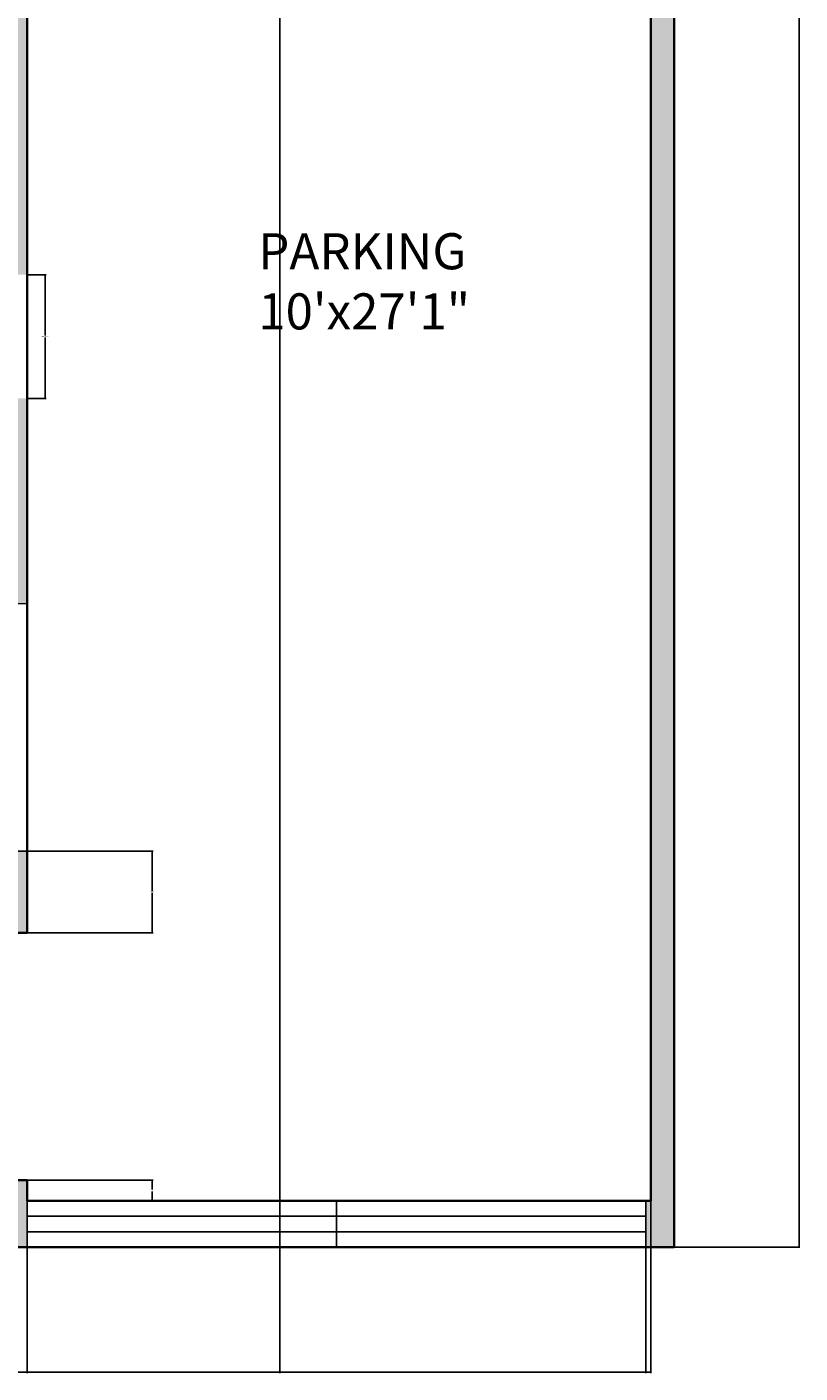
# Model space of a CAD drawing. Units: millimetres. Extents: x 2817 to 5038, y 1110 to 3565.
# Tile 9 of 21: x 3061 to 3211, y 1110 to 1371. Entities that reach past the tile are written whole.
import ezdxf

# ---------------------------------------------------------------- set-up
doc = ezdxf.new("R2010")
doc.units = ezdxf.units.MM
for name, color, linetype, lineweight in [('A-ANNO-DIMS', 2, 'Continuous', 18), ('A-AREA-IDEN', 7, 'Continuous', 18), ('A-WALL', 7, 'Continuous', 35), ('DOOR&WINDOW', 1, 'Continuous', 25)]:
    doc.layers.add(name, color=color, linetype=linetype, lineweight=lineweight)
doc.layers.add('A-WALL-PATT', color=51, linetype='Continuous', lineweight=13, true_color=0xf7f281)
doc.styles.get("Standard").update_dxf_attribs({"font": 'arial.ttf'})
doc.dimstyles.get("Standard").update_dxf_attribs({"dimtxt": 0.18, "dimasz": 0.18, "dimexe": 0.18, "dimexo": 0.0625, "dimgap": 0.09, "dimtad": 0, "dimtih": 1, "dimtoh": 1, "dimdec": 4, "dimzin": 0, "dimdsep": 46, "dimtxsty": 'Standard', "dimcen": 0.09, "dimadec": 0, "dimazin": 0, "dimtfac": 1, "dimtdec": 4, "dimtofl": 0, "dimtmove": 0, "dimatfit": 3, "dimfxl": 1, "dimtolj": 1, "dimtzin": 0, "dimarcsym": 0})

# ---------------------------------------------------------------- blocks, each defined once
blk = doc.blocks.new('WIN-4FT')
for p, q in [((0, 47.85), (9, 48)), ((0, 0), (0, 47.85)), ((3, 0), (3, 47.85)), ((6, 48), (6, 0)), ((9, 48), (9, 0)), ((9, 0), (0, 0))]:
    blk.add_line(p, q)
blk = doc.blocks.new('*D16')
at = {"layer": 'A-ANNO-DIMS', "color": 0, "lineweight": -2, "transparency": 16777216}
for p, q in [((3061.2, 1323.1), (3064.92, 1323.1)), ((3064.74, 1322.92), (3064.74, 1311.28)), ((3064.74, 1299.28), (3064.74, 1310.92)), ((3061.2, 1299.1), (3064.92, 1299.1))]:
    blk.add_line(p, q, dxfattribs=at)
for points in [[(3064.71, 1322.92), (3064.77, 1322.92), (3064.74, 1323.1)], [(3064.71, 1299.28), (3064.77, 1299.28), (3064.74, 1299.1)]]:
    blk.add_solid(points, dxfattribs=at)
at = {"layer": 'Defpoints', "color": 0, "lineweight": -2, "transparency": 16777216}
for p in [(3061.14, 1323.1), (3064.74, 1323.1), (3061.14, 1299.1)]:
    blk.add_point(p, dxfattribs=at)
at = {"layer": 'A-ANNO-DIMS', "color": 0, "transparency": 16777216, "insert": (3064.74, 1311.1), "char_height": 0.18, "attachment_point": 5}
blk.add_mtext('\\A1;WIN. 24 TYP.', dxfattribs=at)
blk = doc.blocks.new('*D27')
at = {"layer": 'A-ANNO-DIMS', "color": 0, "lineweight": -2, "transparency": 16777216}
for p, q in [((3186.8, 1614.44), (3211.17, 1614.44)), ((3210.99, 1614.26), (3210.99, 1374.62)), ((3210.99, 1134.62), (3210.99, 1374.25)), ((3186.8, 1134.44), (3211.17, 1134.44))]:
    blk.add_line(p, q, dxfattribs=at)
for points in [[(3210.96, 1614.26), (3211.02, 1614.26), (3210.99, 1614.44)], [(3210.96, 1134.62), (3211.02, 1134.62), (3210.99, 1134.44)]]:
    blk.add_solid(points, dxfattribs=at)
at = {"layer": 'Defpoints', "color": 0, "lineweight": -2, "transparency": 16777216}
for p in [(3186.74, 1614.44), (3210.99, 1614.44), (3186.74, 1134.44)]:
    blk.add_point(p, dxfattribs=at)
at = {"layer": 'A-ANNO-DIMS', "color": 0, "transparency": 16777216, "insert": (3210.99, 1374.44), "char_height": 0.18, "attachment_point": 5}
blk.add_mtext('\\A1;480', dxfattribs=at)
blk = doc.blocks.new('*D28')
at = {"layer": 'A-ANNO-DIMS', "color": 0, "lineweight": -2, "transparency": 16777216}
for p, q in [((2841.74, 1134.37), (2841.74, 1110.01)), ((3061.24, 1134.37), (3061.24, 1110.01)), ((2841.92, 1110.19), (2951.09, 1110.19)), ((3061.06, 1110.19), (2951.89, 1110.19))]:
    blk.add_line(p, q, dxfattribs=at)
for points in [[(2841.92, 1110.22), (2841.92, 1110.16), (2841.74, 1110.19)], [(3061.06, 1110.22), (3061.06, 1110.16), (3061.24, 1110.19)]]:
    blk.add_solid(points, dxfattribs=at)
at = {"layer": 'Defpoints', "color": 0, "lineweight": -2, "transparency": 16777216}
for p in [(2841.74, 1134.44), (3061.24, 1134.44), (3061.24, 1110.19)]:
    blk.add_point(p, dxfattribs=at)
at = {"layer": 'A-ANNO-DIMS', "color": 0, "transparency": 16777216, "insert": (2951.49, 1110.19), "char_height": 0.18, "attachment_point": 5}
blk.add_mtext('\\A1;219.5', dxfattribs=at)
blk = doc.blocks.new('*D29')
at = {"layer": 'A-ANNO-DIMS', "color": 0, "lineweight": -2, "transparency": 16777216}
for p, q in [((3061.24, 1134.37), (3061.24, 1110.01)), ((3181.24, 1134.37), (3181.24, 1110.01)), ((3061.42, 1110.19), (3120.96, 1110.19)), ((3181.06, 1110.19), (3121.52, 1110.19))]:
    blk.add_line(p, q, dxfattribs=at)
for points in [[(3061.42, 1110.22), (3061.42, 1110.16), (3061.24, 1110.19)], [(3181.06, 1110.22), (3181.06, 1110.16), (3181.24, 1110.19)]]:
    blk.add_solid(points, dxfattribs=at)
at = {"layer": 'Defpoints', "color": 0, "lineweight": -2, "transparency": 16777216}
for p in [(3061.24, 1134.44), (3181.24, 1134.44), (3181.24, 1110.19)]:
    blk.add_point(p, dxfattribs=at)
at = {"layer": 'A-ANNO-DIMS', "color": 0, "transparency": 16777216, "insert": (3121.24, 1110.19), "char_height": 0.18, "attachment_point": 5}
blk.add_mtext('\\A1;120', dxfattribs=at)
blk = doc.blocks.new('*D37')
at = {"layer": 'A-ANNO-DIMS', "color": 0, "lineweight": -2, "transparency": 16777216}
for p, q in [((3110.24, 1473.37), (3110.24, 1110.01)), ((3182.24, 1473.37), (3182.24, 1110.01)), ((3110.42, 1110.19), (3146.02, 1110.19)), ((3182.06, 1110.19), (3146.46, 1110.19))]:
    blk.add_line(p, q, dxfattribs=at)
for points in [[(3110.42, 1110.22), (3110.42, 1110.16), (3110.24, 1110.19)], [(3182.06, 1110.22), (3182.06, 1110.16), (3182.24, 1110.19)]]:
    blk.add_solid(points, dxfattribs=at)
at = {"layer": 'Defpoints', "color": 0, "lineweight": -2, "transparency": 16777216}
for p in [(3110.24, 1473.44), (3182.24, 1473.44), (3182.24, 1110.19)]:
    blk.add_point(p, dxfattribs=at)
at = {"layer": 'A-ANNO-DIMS', "color": 0, "transparency": 16777216, "insert": (3146.24, 1110.19), "char_height": 0.18, "attachment_point": 5}
blk.add_mtext('\\A1;72', dxfattribs=at)
blk = doc.blocks.new('*D48')
at = {"layer": 'A-ANNO-DIMS', "color": 0, "lineweight": -2, "transparency": 16777216}
for p, q in [((3061.3, 1211.29), (3085.67, 1211.29)), ((3085.49, 1211.11), (3085.49, 1203.54)), ((3085.49, 1195.62), (3085.49, 1203.18)), ((3061.3, 1195.44), (3085.67, 1195.44))]:
    blk.add_line(p, q, dxfattribs=at)
for points in [[(3085.46, 1211.11), (3085.52, 1211.11), (3085.49, 1211.29)], [(3085.46, 1195.62), (3085.52, 1195.62), (3085.49, 1195.44)]]:
    blk.add_solid(points, dxfattribs=at)
at = {"layer": 'Defpoints', "color": 0, "lineweight": -2, "transparency": 16777216}
for p in [(3061.24, 1211.29), (3061.24, 1195.44), (3085.49, 1195.44)]:
    blk.add_point(p, dxfattribs=at)
at = {"layer": 'A-ANNO-DIMS', "color": 0, "transparency": 16777216, "insert": (3085.49, 1203.36), "char_height": 0.18, "attachment_point": 5}
blk.add_mtext('\\A1;15.854', dxfattribs=at)
blk = doc.blocks.new('*D50')
at = {"layer": 'A-ANNO-DIMS', "color": 0, "lineweight": -2, "transparency": 16777216}
for p, q in [((3061.301815, 1147.435717), (3085.669315, 1147.435717)), ((3085.489315, 1147.255717), (3085.489315, 1145.615717)), ((3085.489315, 1143.615717), (3085.489315, 1145.255717)), ((3061.301815, 1143.435717), (3085.669315, 1143.435717))]:
    blk.add_line(p, q, dxfattribs=at)
for points in [[(3085.459315, 1147.255717), (3085.519315, 1147.255717), (3085.489315, 1147.435717)], [(3085.459315, 1143.615717), (3085.519315, 1143.615717), (3085.489315, 1143.435717)]]:
    blk.add_solid(points, dxfattribs=at)
at = {"layer": 'Defpoints', "color": 0, "lineweight": -2, "transparency": 16777216}
for p in [(3061.239315, 1147.435717), (3061.239315, 1143.435717), (3085.489315, 1143.435717)]:
    blk.add_point(p, dxfattribs=at)
at = {"layer": 'A-ANNO-DIMS', "color": 0, "transparency": 16777216, "insert": (3085.489315, 1145.435717), "char_height": 0.18, "attachment_point": 5}
blk.add_mtext('\\A1;4', dxfattribs=at)

msp = doc.modelspace()

# ---------------------------------------------------------------- hatches: boundary and pattern name
at = {"layer": 'A-WALL-PATT'}
h = msp.add_hatch(color=256, dxfattribs=at)
h.dxf.hatch_style = 1
h.paths.add_polyline_path([(3186.7393, 1614.4357), (2841.7393, 1614.4357), (2841.7393, 1568.614), (2850.7393, 1568.7609), (2850.7393, 1605.4357), (2982.7393, 1605.4357), (2991.7393, 1605.4357), (3052.2393, 1605.4357), (3052.2393, 1573.7835), (3061.2393, 1573.7835), (3061.2393, 1605.4357), (3182.2393, 1605.4357), (3182.2393, 1143.4357), (3181.2393, 1143.4357), (3181.2393, 1134.4357), (3186.7393, 1134.4357)])
h.paths.add_polyline_path([(3061.2393, 1143.4357), (3061.2393, 1147.4357), (3052.2393, 1147.4357), (3052.2393, 1143.4357), (2850.7393, 1143.4357), (2850.7393, 1145.2996), (2841.7393, 1145.2996), (2841.7393, 1134.4357), (3061.2393, 1134.4357)], flags=17)
h.paths.add_polyline_path([(2850.7393, 1265.4357), (2946.7393, 1265.4357), (2946.7393, 1270.8357), (2946.7393, 1274.4357), (2850.7393, 1274.4357), (2850.7381, 1274.4357), (2850.7381, 1274.2564), (2841.7393, 1274.2564), (2841.7393, 1193.1527), (2850.7393, 1193.2996)], flags=17)
h.paths.add_polyline_path([(3061.2393, 1299.098), (3052.2393, 1299.098), (3052.2393, 1274.4357), (2991.7393, 1274.4357), (2991.7393, 1340.4357), (2982.7393, 1340.4357), (2982.7393, 1274.4357), (2982.7393, 1265.4357), (3052.2393, 1265.4357), (3052.2393, 1259.143), (3061.2393, 1259.2899)], flags=17)
h.paths.add_polyline_path([(3061.2393, 1383.4357), (3052.2393, 1383.4357), (3052.2393, 1379.4357), (2931.7393, 1379.4357), (2922.7393, 1379.4357), (2850.7393, 1379.4357), (2850.7381, 1379.4357), (2850.7381, 1379.3646), (2841.7393, 1379.3646), (2841.7393, 1322.1095), (2850.7393, 1322.2564), (2850.7393, 1370.4357), (2982.7393, 1370.4357), (2987.2393, 1370.4357), (3017.2393, 1370.4357), (3052.2393, 1370.4357), (3052.2393, 1323.098), (3061.2393, 1323.098)], flags=17)
h = msp.add_hatch(color=256, dxfattribs=at)
h.dxf.hatch_style = 1
h.paths.add_polyline_path([(3061.2393, 1549.7835), (3052.2393, 1549.7835), (3052.2393, 1509.4357), (2991.7393, 1509.4357), (2991.7393, 1575.4357), (2982.7393, 1575.4357), (2982.7393, 1509.4357), (2982.7393, 1500.4357), (3052.2393, 1500.4357), (3052.2393, 1498.4661), (3061.2393, 1498.613)])
h.paths.add_polyline_path([(2946.7393, 1505.8357), (2946.7393, 1509.4357), (2850.7393, 1509.4357), (2850.7393, 1520.7609), (2841.7393, 1520.7609), (2841.7393, 1427.2177), (2850.7393, 1427.3646), (2850.7393, 1500.4357), (2922.7393, 1500.4357), (2931.7393, 1500.4357), (2946.7393, 1500.4357)])
h.paths.add_polyline_path([(3061.2393, 1450.613), (3052.2393, 1450.613), (3052.2393, 1431.4357), (3059.4393, 1431.4357), (3061.2393, 1431.4357)])
h.paths.add_polyline_path([(3061.2393, 1211.2899), (3052.2393, 1211.2899), (3052.2393, 1195.4357), (3059.4393, 1195.4357), (3061.2393, 1195.4357)])

# ---------------------------------------------------------------- linework, layer by layer
at = {"layer": 'A-WALL'}
for p, q in [((3186.7393, 1614.4357), (3186.7393, 1134.4357)), ((3182.2393, 1605.4357), (3182.2393, 1143.4357)), ((3061.2393, 1383.4357), (3061.2393, 1195.4357)), ((3052.2393, 1195.4357), (3061.2393, 1195.4357)), ((3052.2393, 1147.4357), (3061.2393, 1147.4357)), ((3061.2393, 1147.4357), (3061.2393, 1143.4357)), ((3182.2393, 1143.4357), (3061.2393, 1143.4357)), ((3186.7393, 1134.4357), (2841.7393, 1134.4357))]:
    msp.add_line(p, q, dxfattribs=at)
at = {"layer": 'DOOR&WINDOW'}
for p, q in [((3061.2393, 1143.4357), (3181.2393, 1143.4357)), ((3061.2393, 1134.4357), (3061.2393, 1143.4357)), ((3121.2393, 1134.4357), (3121.2393, 1143.4357)), ((3181.2393, 1143.4357), (3181.2393, 1134.4357)), ((3061.2393, 1140.4357), (3181.2393, 1140.4357)), ((3181.2393, 1137.4357), (3061.2393, 1137.4357)), ((3181.2393, 1134.4357), (3061.2393, 1134.4357))]:
    msp.add_line(p, q, dxfattribs=at)

# ---------------------------------------------------------------- block references
msp.add_blockref('WIN-4FT', (3052.2393, 1211.2898), dxfattribs=at)

# ---------------------------------------------------------------- texts
at = {"layer": 'A-AREA-IDEN', "insert": (3106.0737, 1331.1453), "char_height": 7, "attachment_point": 1}
msp.add_mtext_dynamic_manual_height_columns('PARKING\\P10\'x27\'1"', width=42.068425, gutter_width=12.5, heights=[0], dxfattribs=at)

# ---------------------------------------------------------------- dimensions: what is measured, and where the dimension line sits
at = {"layer": 'A-ANNO-DIMS'}
for base, p1, p2, angle, override, picture, middle in [((3210.9893, 1614.4357), (3186.7393, 1134.4357), (3186.7393, 1614.4357), 90, {"dimdec": 0, "dimlfac": 1, "dimrnd": 0, "dimzin": 0, "dimdsep": 46, "dimlunit": 2}, '*D27', (3210.9893, 1374.4357)), ((3085.4893, 1195.4357), (3061.2393, 1211.2899), (3061.2393, 1195.4357), 270, {"dimdec": 3, "dimlfac": 1, "dimrnd": 0, "dimzin": 0, "dimdsep": 46, "dimlunit": 2}, '*D48', (3085.4893, 1203.3628)), ((3085.4893, 1143.4357), (3061.2393, 1147.4357), (3061.2393, 1143.4357), 270, {"dimdec": 0, "dimlfac": 1, "dimrnd": 0, "dimzin": 0, "dimdsep": 46, "dimlunit": 2}, '*D50', (3085.4893, 1145.4357))]:
    dim = msp.add_linear_dim(base=base, p1=p1, p2=p2, angle=angle, dimstyle='Standard', override=override, dxfattribs=at)
    dim.commit()
    dim.dimension.update_dxf_attribs({"geometry": picture, "text_midpoint": middle})
for base, p1, p2, override, picture, middle in [((3182.2393, 1110.1857), (3110.2393, 1473.4357), (3182.2393, 1473.4357), {"dimdec": 0, "dimlfac": 1, "dimrnd": 0, "dimzin": 0, "dimdsep": 46, "dimlunit": 2}, '*D37', (3146.2393, 1110.1857)), ((3061.2393, 1110.1857), (2841.7393, 1134.4357), (3061.2393, 1134.4357), {"dimdec": 1, "dimlfac": 1, "dimrnd": 0, "dimzin": 0, "dimdsep": 46, "dimlunit": 2}, '*D28', (2951.4893, 1110.1857)), ((3181.2393, 1110.1857), (3061.2393, 1134.4357), (3181.2393, 1134.4357), {"dimdec": 0, "dimlfac": 1, "dimrnd": 0, "dimzin": 0, "dimdsep": 46, "dimlunit": 2}, '*D29', (3121.2393, 1110.1857))]:
    dim = msp.add_linear_dim(base=base, p1=p1, p2=p2, dimstyle='Standard', override=override, dxfattribs=at)
    dim.commit()
    dim.dimension.update_dxf_attribs({"geometry": picture, "text_midpoint": middle})
dim = msp.add_linear_dim(base=(3064.7378, 1323.098), p1=(3061.1378, 1299.098), p2=(3061.1378, 1323.098), angle=90, text='WIN. <> TYP.', dimstyle='Standard', override={"dimdec": 0, "dimlfac": 1, "dimrnd": 0, "dimzin": 0, "dimdsep": 46, "dimlunit": 2}, dxfattribs=at)
dim.commit()
dim.dimension.update_dxf_attribs({"geometry": '*D16', "text_midpoint": (3064.7378, 1311.098)})

doc.saveas('drawing.dxf')
